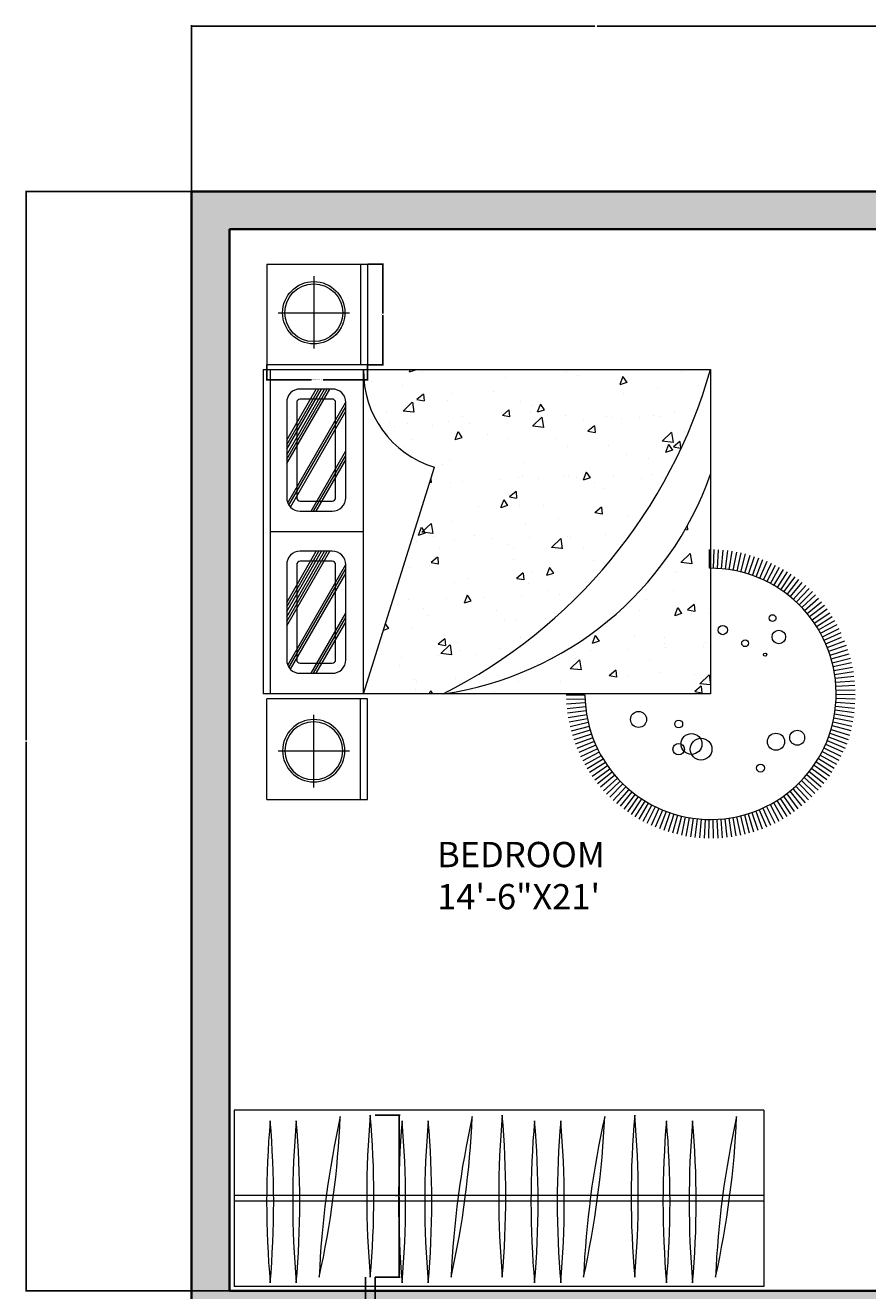
# Model space of a CAD drawing. Units: inches. Extents: x -9 to 646, y -802 to 47.
# Tile 15 of 17: x -9 to 191, y -253 to 47. Entities that reach past the tile are written whole.
import ezdxf

# ---------------------------------------------------------------- set-up
doc = ezdxf.new("R2010")
doc.units = ezdxf.units.IN
doc.header["$MEASUREMENT"] = 0
for name, color, linetype, lineweight in [('A-ANNO-DIMS', 2, 'Continuous', 18), ('A-AREA-IDEN', 7, 'Continuous', 18), ('A-FLOR-CASE', 8, 'Continuous', 18), ('A-FURN', 8, 'Continuous', 15), ('A-FURN-PATT', 252, 'Continuous', 9), ('A-WALL', 7, 'Continuous', 35), ('A-WALL-PATT', 5, 'Continuous', 9)]:
    doc.layers.add(name, color=color, linetype=linetype, lineweight=lineweight)
doc.styles.get("Standard").update_dxf_attribs({"font": 'arial.ttf'})
doc.dimstyles.get("Standard").update_dxf_attribs({"dimtxt": 0.18, "dimasz": 0.18, "dimexe": 0.18, "dimexo": 0.0625, "dimgap": 0.09, "dimtad": 0, "dimtih": 1, "dimtoh": 1, "dimdec": 0, "dimzin": 0, "dimdsep": 46, "dimlunit": 3, "dimtxsty": 'Standard', "dimcen": 0.09, "dimadec": 0, "dimazin": 0, "dimtfac": 1, "dimtdec": 0, "dimtofl": 0, "dimtmove": 0, "dimatfit": 3, "dimfxl": 1, "dimtolj": 1, "dimtzin": 0, "dimarcsym": 0})

# ---------------------------------------------------------------- blocks, each defined once
blk = doc.blocks.new('NIGHTSTAND-24')
for p, q in [((0, 23.9), (23.9, 23.9)), ((0, 23.9), (0, 0)), ((11.11, 21.04), (11.11, 3.84)), ((22.23, 23.9), (22.23, 0)), ((23.9, 23.9), (23.9, 0)), ((2.63, 12.34), (19.6, 12.34)), ((23.9, 0), (0, 0))]:
    blk.add_line(p, q)
for radius in [7.4, 6.87]:
    blk.add_circle((11.11, 12.34), radius)
blk = doc.blocks.new('CLOSET-GARMENT-LONG')
for centre, start, end in [((220.53, 19.21), 175.0028, 184.9972), ((220.53, 19.21), 175.0028, 184.9972), ((-218.85, 19.21), 355.0028, 4.9972), ((-218.85, 19.21), 355.0028, 4.9972)]:
    blk.add_arc(centre, 220.53, start, end)
blk = doc.blocks.new('*D17')
at = {"layer": 'A-ANNO-DIMS', "color": 0, "lineweight": -2, "transparency": 16777216}
for p, q in [((74, -211.4), (79.88, -211.4)), ((79.7, -211.58), (79.7, -230.43)), ((79.7, -249.64), (79.7, -230.8)), ((74, -249.82), (79.88, -249.82))]:
    blk.add_line(p, q, dxfattribs=at)
at = {"layer": 'A-ANNO-DIMS', "color": 0, "transparency": 16777216}
for points in [[(79.67, -211.58), (79.73, -211.58), (79.7, -211.4)], [(79.67, -249.64), (79.73, -249.64), (79.7, -249.82)]]:
    blk.add_solid(points, dxfattribs=at)
at = {"layer": 'Defpoints', "color": 0, "transparency": 16777216}
for p in [(73.94, -211.4), (79.7, -211.4), (73.94, -249.82)]:
    blk.add_point(p, dxfattribs=at)
at = {"layer": 'A-ANNO-DIMS', "color": 0, "transparency": 16777216, "insert": (79.7, -230.61), "char_height": 0.18, "attachment_point": 5}
blk.add_mtext('\\A1;GARMENT 38 TYP.', dxfattribs=at)
blk = doc.blocks.new('*D18')
at = {"layer": 'A-ANNO-DIMS', "color": 0, "lineweight": -2, "transparency": 16777216}
for p, q in [((71.7, -249.89), (71.7, -255.77)), ((73.94, -249.89), (73.94, -255.77)), ((71.88, -255.59), (72.36, -255.59)), ((73.76, -255.59), (73.28, -255.59))]:
    blk.add_line(p, q, dxfattribs=at)
at = {"layer": 'A-ANNO-DIMS', "color": 0, "transparency": 16777216}
for points in [[(71.88, -255.56), (71.88, -255.62), (71.7, -255.59)], [(73.76, -255.56), (73.76, -255.62), (73.94, -255.59)]]:
    blk.add_solid(points, dxfattribs=at)
at = {"layer": 'Defpoints', "color": 0, "transparency": 16777216}
for p in [(71.7, -249.82), (73.94, -249.82), (73.94, -255.59)]:
    blk.add_point(p, dxfattribs=at)
at = {"layer": 'A-ANNO-DIMS', "color": 0, "transparency": 16777216, "insert": (72.82, -255.59), "char_height": 0.18, "attachment_point": 5}
blk.add_mtext('\\A1;2 TYP.', dxfattribs=at)
blk = doc.blocks.new('*D47')
at = {"layer": 'A-ANNO-DIMS', "color": 0, "lineweight": -2, "transparency": 16777216}
for p, q in [((48.29, -33.28), (48.29, -36.98)), ((72.19, -33.28), (72.19, -36.98)), ((48.47, -36.8), (58.86, -36.8)), ((72.01, -36.8), (61.62, -36.8))]:
    blk.add_line(p, q, dxfattribs=at)
at = {"layer": 'A-ANNO-DIMS', "color": 0, "transparency": 16777216}
for points in [[(48.47, -36.77), (48.47, -36.83), (48.29, -36.8)], [(72.01, -36.77), (72.01, -36.83), (72.19, -36.8)]]:
    blk.add_solid(points, dxfattribs=at)
at = {"layer": 'Defpoints', "color": 0, "transparency": 16777216}
for p in [(48.29, -33.22), (72.19, -33.22), (72.19, -36.8)]:
    blk.add_point(p, dxfattribs=at)
at = {"layer": 'A-ANNO-DIMS', "color": 0, "transparency": 16777216, "insert": (60.24, -36.8), "char_height": 0.18, "attachment_point": 5}
blk.add_mtext('\\A1;NIGHTSTAND 24 TYP.', dxfattribs=at)
blk = doc.blocks.new('*D48')
at = {"layer": 'A-ANNO-DIMS', "color": 0, "lineweight": -2, "transparency": 16777216}
for p, q in [((72.25, -9.32), (75.96, -9.32)), ((75.78, -9.5), (75.78, -21.09)), ((75.78, -33.04), (75.78, -21.45)), ((72.25, -33.22), (75.96, -33.22))]:
    blk.add_line(p, q, dxfattribs=at)
at = {"layer": 'A-ANNO-DIMS', "color": 0, "transparency": 16777216}
for points in [[(75.75, -9.5), (75.81, -9.5), (75.78, -9.32)], [(75.75, -33.04), (75.81, -33.04), (75.78, -33.22)]]:
    blk.add_solid(points, dxfattribs=at)
at = {"layer": 'Defpoints', "color": 0, "transparency": 16777216}
for p in [(72.19, -9.32), (75.78, -9.32), (72.19, -33.22)]:
    blk.add_point(p, dxfattribs=at)
at = {"layer": 'A-ANNO-DIMS', "color": 0, "transparency": 16777216, "insert": (75.78, -21.27), "char_height": 0.18, "attachment_point": 5}
blk.add_mtext('\\A1;24 TYP.', dxfattribs=at)
blk = doc.blocks.new('*D51')
at = {"layer": 'A-ANNO-DIMS', "color": 0, "lineweight": -2, "transparency": 16777216}
for p, q in [((30.37, 7.99), (30.37, 47.36)), ((30.55, 47.18), (126.09, 47.18)), ((222.19, 47.18), (126.65, 47.18)), ((222.37, 7.99), (222.37, 47.36))]:
    blk.add_line(p, q, dxfattribs=at)
at = {"layer": 'A-ANNO-DIMS', "color": 0, "transparency": 16777216}
for points in [[(30.55, 47.21), (30.55, 47.15), (30.37, 47.18)], [(222.19, 47.21), (222.19, 47.15), (222.37, 47.18)]]:
    blk.add_solid(points, dxfattribs=at)
at = {"layer": 'Defpoints', "color": 0, "transparency": 16777216}
for p in [(222.37, 47.18), (30.37, 7.93), (222.37, 7.93)]:
    blk.add_point(p, dxfattribs=at)
at = {"layer": 'A-ANNO-DIMS', "color": 0, "transparency": 16777216, "insert": (126.37, 47.18), "char_height": 0.18, "attachment_point": 5}
blk.add_mtext('\\A1;192', dxfattribs=at)
blk = doc.blocks.new('*D54')
at = {"layer": 'A-ANNO-DIMS', "color": 0, "lineweight": -2, "transparency": 16777216}
for p, q in [((30.31, 7.93), (-9.06, 7.93)), ((-8.88, 7.75), (-8.88, -122.39)), ((-8.88, -252.89), (-8.88, -122.75)), ((39.31, -253.07), (-9.06, -253.07))]:
    blk.add_line(p, q, dxfattribs=at)
at = {"layer": 'A-ANNO-DIMS', "color": 0, "transparency": 16777216}
for points in [[(-8.91, 7.75), (-8.85, 7.75), (-8.88, 7.93)], [(-8.91, -252.89), (-8.85, -252.89), (-8.88, -253.07)]]:
    blk.add_solid(points, dxfattribs=at)
at = {"layer": 'Defpoints', "color": 0, "transparency": 16777216}
for p in [(30.37, 7.93), (-8.88, -253.07), (39.37, -253.07)]:
    blk.add_point(p, dxfattribs=at)
at = {"layer": 'A-ANNO-DIMS', "color": 0, "transparency": 16777216, "insert": (-8.88, -122.57), "char_height": 0.18, "attachment_point": 5}
blk.add_mtext('\\A1;261', dxfattribs=at)

msp = doc.modelspace()

# ---------------------------------------------------------------- hatches: boundary and pattern name
at = {"layer": 'A-FURN-PATT'}
h = msp.add_hatch(dxfattribs=at)
h.set_pattern_fill('AR-CONC', color=256, scale=0.106234, angle=270, style=0)
h.set_pattern_definition([(220, (6076.148, 873.132), (1.693277, -19.354254), [2.02376, -22.26139]), (275, (6076.148, 873.132), (-20.29676, 3.743996), [1.61901, -17.80911]), (169.549, (6076.289, 871.52), (-18.60339, -15.61033), [1.71993, -18.91926]), (223.8158, (6070.75, 873.132), (4.46634, -28.79788), [3.03564, -33.39208]), (173.3644, (6071.123, 870.732), (-26.28507, -25.22046), [2.5799, -28.37889]), (278.816, (6070.75, 873.132), (-26.28502, -25.2205), [2.42852, -26.71367]), (249, (6072.1, 870.434), (10.8641, -16.106695), [2.02376, -22.26139]), (304, (6072.1, 870.434), (-19.56707, -6.56549), [1.61901, -17.80911]), (198.5486, (6073.006, 869.092), (-8.703014, -22.672143), [1.71993, -18.91926]), (232.5, (6076.148, 873.132), (-8.982642, -0.3281155), [0, -17.593244, 0, -18.078947, 0, -17.87657]), (262.5, (6076.148, 873.132), (-10.64261, -7.098538), [0, -10.307698, 0, -17.188491, 0, -6.813334]), (302.5, (6076.148, 879.1495), (0.608589, -14.404367), [0, -6.745876, 0, -21.047132, 0, -27.927925]), (312.5, (6076.148, 881.848), (-2.701165, -15.736394), [0, -8.769638, 0, -13.977454, 0, -19.832874])])
edge = h.paths.add_edge_path()
edge.add_ellipse((94.96, -34.84), major_axis=(-16.79, -16.79), ratio=1, start_angle=-43.8468, end_angle=28.0453, ccw=False)
edge.add_line((71.22, -35.32), (71.22, -34.36))
edge.add_line((71.22, -34.36), (153.6, -34.36))
edge.add_ellipse((34.11, -0.53), major_axis=(-87.81, -87.81), ratio=1, start_angle=71.7955, end_angle=119.1914, ccw=False)
edge.add_line((90.1, -111.38), (71.22, -111.38))
edge.add_line((71.22, -111.38), (88.04, -57.56))
edge = h.paths.add_edge_path()
edge.add_line((153.6, -59.21), (153.6, -111.38))
edge.add_line((153.6, -111.38), (90.1, -111.38))
edge.add_ellipse((78.69, -32.76), major_axis=(-56.18, 56.18), ratio=1, start_angle=143.2583, end_angle=205.5572)
h = msp.add_hatch(dxfattribs=at)
h.set_pattern_fill('ANSI31', color=256, scale=4.24079, angle=15.0416, style=0)
h.paths.add_polyline_path([(52.97, -54.34), (52.97, -56.98), (63.33, -38.99), (61.81, -38.99)])
h = msp.add_hatch(dxfattribs=at)
h.set_pattern_fill('ANSI31', color=256, scale=4.26443, angle=15.0416, style=0)
h.paths.add_polyline_path([(52.97, -50.89), (52.97, -53.53), (61.35, -38.99), (59.83, -38.99)])
h = msp.add_hatch(dxfattribs=at)
h.set_pattern_fill('ANSI31', color=256, scale=4.24573, angle=15.0416, style=0)
h.paths.add_polyline_path([(53.16, -65.87), (53.17, -65.92), (53.21, -66.01), (53.25, -66.11), (53.29, -66.2), (53.34, -66.29), (53.39, -66.39), (53.45, -66.47), (53.5, -66.56), (53.56, -66.65), (53.62, -66.73), (53.69, -66.81), (53.76, -66.89), (53.83, -66.97), (53.9, -67.05), (53.96, -67.11), (66.98, -44.53), (66.98, -42.18), (66.98, -42.07), (66.97, -41.97), (66.97, -41.91)])
h = msp.add_hatch(dxfattribs=at)
h.set_pattern_fill('ANSI31', color=256, scale=4.24231, angle=15.0416, style=0)
h.paths.add_polyline_path([(58.6, -67.98), (60.12, -67.98), (66.98, -56.08), (66.98, -53.44)])
h = msp.add_hatch(dxfattribs=at)
h.set_pattern_fill('ANSI31', color=256, scale=4.24752, angle=15.0416, style=0)
h.paths.add_polyline_path([(52.97, -92.85), (52.97, -95.49), (63.33, -77.5), (61.81, -77.5)])
h = msp.add_hatch(dxfattribs=at)
h.set_pattern_fill('ANSI31', color=256, scale=4.24153, angle=15.0416, style=0)
h.paths.add_polyline_path([(52.97, -89.4), (52.97, -92.04), (61.35, -77.5), (59.83, -77.5)])
h = msp.add_hatch(dxfattribs=at)
h.set_pattern_fill('ANSI31', color=256, scale=4.2511, angle=15.0416, style=0)
h.paths.add_polyline_path([(53.15, -104.38), (53.22, -104.54), (53.3, -104.73), (53.4, -104.91), (53.51, -105.09), (53.63, -105.25), (53.76, -105.41), (53.9, -105.56), (53.96, -105.62), (66.98, -83.04), (66.98, -80.69), (66.97, -80.47), (66.97, -80.42)])
h = msp.add_hatch(dxfattribs=at)
h.set_pattern_fill('ANSI31', color=256, scale=4.24801, angle=15.0416, style=0)
h.paths.add_polyline_path([(58.6, -106.49), (60.12, -106.49), (66.98, -94.59), (66.98, -91.95)])
at = {"layer": 'A-WALL-PATT'}
h = msp.add_hatch(color=256, dxfattribs=at)
h.dxf.hatch_style = 1
h.paths.add_polyline_path([(73.4, -418.07), (63.37, -418.07), (63.37, -487.07), (63.35, -496.07), (67.87, -496.07), (67.87, -427.07), (73.4, -427.07)])
h.paths.add_polyline_path([(73.87, -487.07), (67.87, -487.07), (67.87, -496.07), (73.87, -496.07)])
h.paths.add_polyline_path([(39.37, -496.07), (39.35, -496.07), (39.35, -487.07), (30.37, -487.07), (30.37, -646.07), (69.62, -646.07), (69.62, -637.07), (39.37, -637.07)])
h.paths.add_polyline_path([(158.27, -637.07), (105.62, -637.07), (105.62, -646.07), (158.27, -646.07)])
h.paths.add_polyline_path([(286.47, -637.07), (194.27, -637.07), (194.27, -646.07), (286.47, -646.07)])
h.paths.add_polyline_path([(357.37, -552.07), (352.87, -552.07), (348.37, -552.07), (348.37, -637.07), (322.47, -637.07), (322.47, -646.07), (357.37, -646.07)])
h.paths.add_polyline_path([(357.37, -459.07), (352.87, -459.07), (348.37, -459.07), (348.37, -526.07), (357.37, -526.07), (357.37, -520.07), (363.37, -520.07), (363.37, -511.07), (357.37, -511.07)], flags=17)
h.paths.add_polyline_path([(39.37, -262.07), (213.37, -262.07), (213.37, -268.07), (222.37, -268.07), (222.37, -247.07), (213.37, -247.07), (213.37, -253.07), (39.37, -253.07), (39.37, -1.07), (222.37, -1.07), (222.37, 7.93), (30.37, 7.93), (30.37, -427.07), (39.36, -427.07), (39.36, -418.07)])
h.paths.add_polyline_path([(570.37, -149.32), (561.37, -149.32), (561.37, -161.07), (433.37, -161.07), (433.37, -165.57), (433.37, -170.07), (438.37, -170.07), (438.37, -176.07), (447.37, -176.07), (447.37, -170.07), (561.37, -170.07), (561.37, -229.57), (570.37, -229.57)])
h.paths.add_polyline_path([(570.37, -289.57), (561.37, -289.57), (561.37, -349.07), (479.37, -349.07), (479.37, -353.57), (479.37, -358.07), (561.37, -358.07), (561.37, -418.07), (447.37, -418.07), (447.37, -358.07), (453.37, -358.07), (453.37, -349.07), (447.37, -349.07), (447.37, -202.07), (442.87, -202.07), (438.37, -202.07), (438.37, -427.07), (561.37, -427.07), (561.37, -451.07), (570.37, -451.07)])
h.paths.add_polyline_path([(570.37, -496.07), (570.37, -487.07), (561.37, -487.07), (561.37, -511.07), (411.37, -511.07), (411.37, -515.57), (411.37, -520.07), (570.37, -520.07)])

# ---------------------------------------------------------------- linework, layer by layer
at = {"layer": 'A-FLOR-CASE'}
for p, q in [((166.25, -210.17), (40.52, -210.17)), ((40.52, -210.17), (40.52, -252.08)), ((166.25, -210.17), (40.52, -210.17)), ((166.25, -210.17), (166.25, -252.08)), ((166.25, -210.17), (166.25, -252.08)), ((166.25, -230.43), (40.52, -230.43)), ((166.25, -230.43), (40.52, -230.43)), ((166.25, -231.83), (40.52, -231.83)), ((166.25, -231.83), (40.52, -231.83)), ((166.25, -252.08), (40.52, -252.08)), ((166.25, -252.08), (48.51, -252.08))]:
    msp.add_line(p, q, dxfattribs=at)
at = {"layer": 'A-FURN'}
for p, q in [((47.37, -34.36), (47.37, -111.38)), ((47.37, -34.36), (153.6, -34.36)), ((49.11, -111.38), (49.11, -34.36)), ((71.22, -111.38), (71.22, -34.36)), ((153.6, -34.36), (153.6, -111.38)), ((71.22, -111.38), (88.04, -57.56)), ((71.22, -72.87), (49.11, -72.87)), ((153.34, -81.56), (153.34, -77.12)), ((154.29, -81.57), (154.43, -77.13)), ((155.23, -81.6), (155.51, -77.18)), ((156.17, -81.67), (156.59, -77.25)), ((157.11, -81.77), (157.67, -77.37)), ((158.04, -81.89), (158.74, -77.51)), ((158.97, -82.05), (159.81, -77.69)), ((159.9, -82.23), (160.87, -77.9)), ((160.82, -82.45), (161.93, -78.15)), ((161.73, -82.69), (162.97, -78.43)), ((162.63, -82.96), (164.01, -78.74)), ((163.53, -83.26), (165.04, -79.09)), ((164.41, -83.59), (166.05, -79.47)), ((165.28, -83.94), (167.06, -79.88)), ((166.15, -84.33), (168.05, -80.32)), ((167, -84.74), (169.02, -80.79)), ((167.83, -85.17), (169.98, -81.29)), ((168.65, -85.64), (170.92, -81.83)), ((169.46, -86.12), (171.85, -82.39)), ((170.25, -86.64), (172.76, -82.98)), ((171.02, -87.18), (173.65, -83.6)), ((171.78, -87.74), (174.52, -84.25)), ((172.52, -88.33), (175.36, -84.92)), ((173.24, -88.94), (176.19, -85.62)), ((173.94, -89.57), (176.99, -86.35)), ((174.62, -90.22), (177.77, -87.1)), ((175.28, -90.9), (178.53, -87.88)), ((175.91, -91.59), (179.26, -88.68)), ((176.53, -92.31), (179.96, -89.5)), ((177.12, -93.04), (180.64, -90.35)), ((177.69, -93.8), (181.29, -91.21)), ((178.23, -94.57), (181.92, -92.1)), ((178.75, -95.35), (182.51, -93)), ((179.25, -96.16), (183.08, -93.93)), ((179.72, -96.98), (183.62, -94.87)), ((180.16, -97.81), (184.13, -95.82)), ((180.57, -98.66), (184.6, -96.8)), ((180.96, -99.52), (184.69, -97.94)), ((181.32, -100.39), (185.47, -98.78)), ((181.66, -101.27), (185.86, -99.8)), ((181.96, -102.16), (186.21, -100.82)), ((182.24, -103.06), (186.54, -101.85)), ((182.49, -103.97), (186.83, -102.9)), ((182.71, -104.89), (187.08, -103.95)), ((182.9, -105.81), (187.31, -105.02)), ((183.06, -106.74), (187.5, -106.08)), ((183.2, -107.68), (187.65, -107.16)), ((183.3, -108.61), (187.77, -108.24)), ((183.37, -109.55), (187.86, -109.32)), ((183.41, -110.5), (187.92, -110.4)), ((153.6, -111.38), (47.37, -111.38)), ((123.78, -111.64), (119.34, -111.64)), ((123.8, -112.59), (119.37, -112.73)), ((123.85, -113.53), (119.43, -113.81)), ((183.36, -113.32), (187.88, -113.66)), ((183.41, -112.38), (187.92, -112.57)), ((183.43, -111.44), (187.94, -111.49)), ((123.94, -114.47), (119.52, -114.89)), ((124.05, -115.4), (119.65, -115.96)), ((124.19, -116.34), (119.81, -117.03)), ((182.88, -117.06), (187.34, -117.97)), ((183.05, -116.14), (187.53, -116.9)), ((183.18, -115.2), (187.68, -115.82)), ((183.29, -114.26), (187.79, -114.74)), ((124.36, -117.26), (120.01, -118.1)), ((124.56, -118.19), (120.24, -119.16)), ((124.79, -119.1), (120.5, -120.21)), ((125.05, -120.01), (120.79, -121.25)), ((182.21, -119.81), (186.59, -121.14)), ((182.46, -118.9), (186.87, -120.09)), ((182.69, -117.99), (187.12, -119.04)), ((125.34, -120.91), (121.12, -122.29)), ((125.65, -121.79), (121.48, -123.31)), ((126, -122.67), (121.88, -124.32)), ((181.28, -122.48), (185.54, -124.23)), ((181.62, -121.6), (185.92, -123.21)), ((181.93, -120.71), (186.27, -122.18)), ((126.37, -123.54), (122.3, -125.31)), ((126.77, -124.4), (122.76, -126.3)), ((127.19, -125.24), (123.24, -127.26)), ((127.64, -126.07), (123.76, -128.22)), ((179.66, -125.89), (183.52, -128.08)), ((180.11, -125.06), (184.03, -127.13)), ((180.53, -124.21), (184.51, -126.16)), ((180.92, -123.35), (184.97, -125.17)), ((128.12, -126.88), (124.31, -129.15)), ((128.62, -127.68), (124.89, -130.07)), ((129.15, -128.46), (125.49, -130.97)), ((177.62, -129.06), (181.17, -131.72)), ((178.17, -128.29), (181.8, -130.84)), ((178.69, -127.51), (182.4, -129.94)), ((179.19, -126.71), (182.98, -129.02)), ((129.7, -129.22), (126.12, -131.85)), ((130.28, -129.97), (126.78, -132.71)), ((130.88, -130.7), (127.47, -133.54)), ((131.5, -131.41), (128.19, -134.36)), ((132.14, -132.1), (128.92, -135.15)), ((175.2, -131.95), (178.39, -135.04)), ((175.84, -131.26), (179.12, -134.24)), ((176.46, -130.54), (179.83, -133.42)), ((177.05, -129.81), (180.52, -132.58)), ((132.81, -132.77), (129.69, -135.92)), ((133.5, -133.41), (130.48, -136.66)), ((134.2, -134.04), (131.29, -137.38)), ((134.93, -134.64), (132.12, -138.07)), ((171.69, -135.1), (174.35, -138.65)), ((172.43, -134.51), (175.2, -137.98)), ((173.16, -133.9), (176.03, -137.28)), ((173.86, -133.27), (176.84, -136.56)), ((174.54, -132.62), (177.63, -135.81)), ((135.67, -135.22), (132.98, -138.74)), ((136.44, -135.77), (133.85, -139.38)), ((137.22, -136.3), (134.75, -139.99)), ((138.01, -136.81), (135.66, -140.57)), ((138.82, -137.29), (136.59, -141.12)), ((139.65, -137.74), (137.54, -141.65)), ((140.49, -138.17), (138.51, -142.14)), ((166.9, -138.08), (168.84, -142.07)), ((167.73, -137.65), (169.8, -141.57)), ((168.56, -137.19), (170.75, -141.05)), ((169.37, -136.7), (171.68, -140.49)), ((170.16, -136.19), (172.59, -139.9)), ((170.93, -135.66), (173.48, -139.29)), ((141.34, -138.57), (139.49, -142.6)), ((142.21, -138.95), (140.48, -143.03)), ((143.09, -139.29), (141.49, -143.43)), ((143.97, -139.61), (142.51, -143.8)), ((144.87, -139.9), (143.54, -144.13)), ((145.78, -140.16), (144.58, -144.43)), ((146.69, -140.4), (145.63, -144.7)), ((147.61, -140.6), (146.68, -144.94)), ((148.54, -140.78), (147.75, -145.14)), ((149.47, -140.92), (148.82, -145.31)), ((150.41, -141.04), (149.9, -145.44)), ((151.35, -141.12), (150.97, -145.54)), ((152.29, -141.18), (152.06, -145.61)), ((155.12, -141.17), (155.3, -145.6)), ((156.06, -141.11), (156.39, -145.53)), ((157, -141.01), (157.46, -145.43)), ((157.93, -140.89), (158.54, -145.29)), ((158.86, -140.74), (159.61, -145.11)), ((159.79, -140.56), (160.67, -144.91)), ((160.71, -140.35), (161.73, -144.67)), ((161.62, -140.11), (162.78, -144.39)), ((162.53, -139.84), (163.82, -144.09)), ((163.42, -139.55), (164.85, -143.75)), ((164.31, -139.22), (165.86, -143.38)), ((165.18, -138.87), (166.87, -142.97)), ((166.04, -138.49), (167.86, -142.54)), ((153.23, -141.21), (153.14, -145.64)), ((154.18, -141.2), (154.22, -145.64))]:
    msp.add_line(p, q, dxfattribs=at)
for points in [[(52.97, -42.18), (52.97, -64.79, 0.414214), (56.15, -67.98), (63.79, -67.98, 0.414214), (66.98, -64.79), (66.98, -42.18, 0.414214), (63.79, -38.99), (56.15, -38.99, 0.414214)], [(55.36, -42.18), (55.36, -64.79, 0.414214), (56.15, -65.59), (63.79, -65.59, 0.414214), (64.59, -64.79), (64.59, -42.18, 0.414214), (63.79, -41.38), (56.15, -41.38, 0.414214)], [(52.97, -80.69), (52.97, -103.3, 0.414214), (56.15, -106.49), (63.79, -106.49, 0.414214), (66.98, -103.3), (66.98, -80.69, 0.414214), (63.79, -77.5), (56.15, -77.5, 0.414214)], [(55.36, -80.69), (55.36, -103.3, 0.414214), (56.15, -104.1), (63.79, -104.1, 0.414214), (64.59, -103.3), (64.59, -80.69, 0.414214), (63.79, -79.89), (56.15, -79.89, 0.414214)]]:
    msp.add_lwpolyline(points, format="xyb", close=True, dxfattribs=at)
for centre, radius in [((168.32, -93.38), 0.809), ((156.5, -96.22), 1.1), ((161.8, -99.35), 0.809), ((169.81, -97.86), 1.62), ((166.55, -102.06), 0.391), ((136.52, -117.43), 1.9), ((146.04, -118.53), 0.939), ((174.17, -121.79), 1.77), ((146.04, -124.5), 1.36), ((149.07, -123.27), 2.48), ((151.34, -124.5), 2.58), ((169.13, -122.73), 2.03), ((165.45, -128.99), 0.939)]:
    msp.add_circle(centre, radius, dxfattribs=at)
for centre, radius, start, end in [((94.96, -34.84), 23.75, 178.8468, 253.0453), ((34.11, -0.53), 124.19, 296.7955, 344.1914), ((78.69, -32.76), 79.45, 278.2583, 340.5572), ((153.6, -111.38), 29.82, 180.4973, 90.4973)]:
    msp.add_arc(centre, radius, start, end, dxfattribs=at)
at = {"layer": 'A-WALL'}
for p, q in [((30.37, 7.93), (30.37, -646.07)), ((30.37, 7.93), (570.37, 7.93)), ((39.37, -1.07), (213.37, -1.07)), ((39.37, -1.07), (39.37, -253.07)), ((39.37, -253.07), (213.37, -253.07))]:
    msp.add_line(p, q, dxfattribs=at)

# ---------------------------------------------------------------- block references
at = {"layer": 'A-FLOR-CASE'}
for p, rotation in [((49.89, -212.76), 180), ((66.53, -211.85), 172.5051423894902), ((81.21, -212.76), 180), ((97.86, -211.85), 172.5051423894902), ((118.87, -212.76), 180), ((122.62, -249.72), 352.5051423895286), ((136.43, -211.41), 180), ((150.19, -212.76), 180), ((153.95, -249.72), 352.5051423896668)]:
    msp.add_blockref('CLOSET-GARMENT-LONG', p, dxfattribs=dict(at, rotation=rotation))
for p in [(54.41, -251.17), (71.98, -249.82), (85.74, -251.17), (103.31, -249.82), (110.97, -251.17), (142.3, -251.17)]:
    msp.add_blockref('CLOSET-GARMENT-LONG', p, dxfattribs=at)
at = {"layer": 'A-FURN'}
msp.add_blockref('NIGHTSTAND-24', (48.29, -33.22), dxfattribs=at)
at = {"layer": 'A-FURN', "extrusion": (0, 0, -1), "zscale": -1, "rotation": 180}
msp.add_blockref('NIGHTSTAND-24', (-48.29, -112.53), dxfattribs=at)

# ---------------------------------------------------------------- texts
at = {"layer": 'A-AREA-IDEN', "insert": (88.69, -146.52), "char_height": 6, "attachment_point": 1}
msp.add_mtext('BEDROOM\\P14\'-6"X21\'', dxfattribs=at)

# ---------------------------------------------------------------- dimensions: what is measured, and where the dimension line sits
at = {"layer": 'A-ANNO-DIMS'}
dim = msp.add_linear_dim(base=(222.37, 47.18), p1=(30.37, 7.93), p2=(222.37, 7.93), dimstyle='Standard', override={"dimdec": 0, "dimlfac": 1, "dimrnd": 0, "dimzin": 0, "dimdsep": 46, "dimlunit": 2}, dxfattribs=at)
dim.commit()
dim.dimension.update_dxf_attribs({"geometry": '*D51', "text_midpoint": (126.37, 47.18)})
dim = msp.add_linear_dim(base=(-8.88, -253.07), p1=(30.37, 7.93), p2=(39.37, -253.07), angle=90, dimstyle='Standard', override={"dimdec": 0, "dimlfac": 1, "dimrnd": 0, "dimzin": 0, "dimdsep": 46, "dimlunit": 2}, dxfattribs=at)
dim.commit()
dim.dimension.update_dxf_attribs({"geometry": '*D54', "text_midpoint": (-8.88, -122.57)})
for base, p1, p2, text, picture, middle in [((75.78, -9.32), (72.19, -33.22), (72.19, -9.32), '<> TYP.', '*D48', (75.78, -21.27)), ((79.7, -211.4), (73.94, -249.82), (73.94, -211.4), 'GARMENT <> TYP.', '*D17', (79.7, -230.61))]:
    dim = msp.add_linear_dim(base=base, p1=p1, p2=p2, angle=90, text=text, dimstyle='Standard', override={"dimdec": 0, "dimlfac": 1, "dimrnd": 0, "dimzin": 0, "dimdsep": 46, "dimlunit": 2}, dxfattribs=at)
    dim.commit()
    dim.dimension.update_dxf_attribs({"geometry": picture, "text_midpoint": middle})
for base, p1, p2, text, picture, middle in [((72.19, -36.8), (48.29, -33.22), (72.19, -33.22), 'NIGHTSTAND <> TYP.', '*D47', (60.24, -36.8)), ((73.94, -255.59), (71.7, -249.82), (73.94, -249.82), '<> TYP.', '*D18', (72.82, -255.59))]:
    dim = msp.add_linear_dim(base=base, p1=p1, p2=p2, text=text, dimstyle='Standard', override={"dimdec": 0, "dimlfac": 1, "dimrnd": 0, "dimzin": 0, "dimdsep": 46, "dimlunit": 2}, dxfattribs=at)
    dim.commit()
    dim.dimension.update_dxf_attribs({"geometry": picture, "text_midpoint": middle})

doc.saveas('drawing.dxf')
